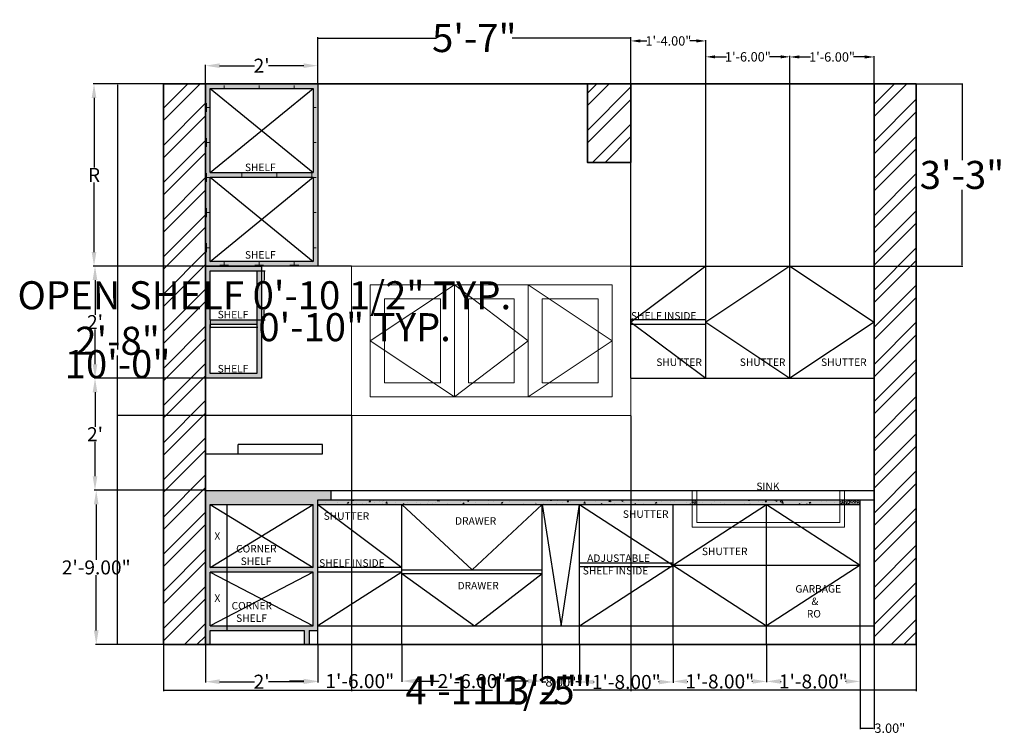
# Model space of a CAD drawing. Units: inches. Extents: x 14 to 1508, y -30 to 806.
# Tile 3 of 4: x 782 to 993, y 297 to 450. Entities that reach past the tile are written whole.
import ezdxf

# ---------------------------------------------------------------- set-up
doc = ezdxf.new("R2010")
doc.units = ezdxf.units.IN
doc.header["$MEASUREMENT"] = 0
for name, color, linetype, lineweight in [('A-ANNO-DIMS', 6, 'Continuous', 18), ('A-ANNO-TEXT', 7, 'Continuous', 18), ('A-ELEV-CASE-BASE', 7, 'Continuous', 25), ('A-ELEV-CASE-PATT', 8, 'Continuous', 13), ('A-ELEV-CASE-UPPR', 7, 'Continuous', 25), ('A-ELEV-CNTR', 7, 'Continuous', 25), ('A-FLOR-FIXT', 8, 'Continuous', 18), ('A-GLAZ', 4, 'Continuous', 18), ('A-WALL', 7, 'Continuous', 35), ('A-WALL-PATT', 8, 'Continuous', 13)]:
    doc.layers.add(name, color=color, linetype=linetype, lineweight=lineweight)
doc.styles.get("Standard").update_dxf_attribs({"font": 'arial.ttf'})
doc.dimstyles.get("Standard").update_dxf_attribs({"dimtxt": 6, "dimasz": 0.18, "dimexe": 0.18, "dimexo": 0.0625, "dimgap": 0.09, "dimtad": 0, "dimtih": 1, "dimtoh": 1, "dimzin": 0, "dimdsep": 46, "dimlunit": 3, "dimtxsty": 'Standard', "dimcen": 0.09, "dimadec": 0, "dimazin": 0, "dimtfac": 1, "dimtofl": 0, "dimtmove": 0, "dimatfit": 3, "dimfxl": 1, "dimtolj": 1, "dimtzin": 0, "dimarcsym": 0})
pattern_1 = [(50, (0, 0), (0.35863009, -0.03137607), [0.0375, -0.4125]), (355, (0, 0), (-0.06937567, 0.37609607), [0.03, -0.33]), (100.451444, (0.0299, -0.0026), (0.28925442, 0.34472), [0.0318701, -0.35057106]), (46.1842, (0, 0.1), (0.53362067, -0.08275964), [0.05625, -0.61875]), (96.635635, (0.04447, 0.0931), (0.46733097, 0.4870593), [0.04780517, -0.52585688]), (351.184164, (0, 0.1), (0.46733097, 0.4870593), [0.045, -0.495]), (21, (0.05, 0.075), (0.29845353, -0.201309445), [0.0375, -0.4125]), (326, (0.05, 0.075), (0.12165767, 0.36257502), [0.03, -0.33]), (71.451445, (0.07487, 0.05822), (0.42011119, 0.16126558), [0.0318701, -0.35057106]), (37.5, (0, 0), (0.006079928, 0.166446927), [0, -0.326, 0, -0.335, 0, -0.33125]), (7.5, (0, 0), (0.13153477, 0.197205856), [0, -0.191, 0, -0.3185, 0, -0.12625]), (327.5, (-0.1115, 0), (0.266911218, -0.011277436), [0, -0.125, 0, -0.39, 0, -0.5175]), (317.5, (-0.1615, 0), (0.291593085, 0.05005249), [0, -0.1625, 0, -0.259, 0, -0.3675])]
pattern_2 = [(50, (0, 0), (3.586301, -0.313761), [0.375, -4.125]), (355, (0, 0), (-0.693757, 3.760961), [0.3, -3.3]), (100.45144, (0.299, -0.026), (2.892544, 3.4472), [0.318701, -3.50571]), (46.1842, (0, 1), (5.336207, -0.827596), [0.5625, -6.1875]), (96.63564, (0.4447, 0.931), (4.67331, 4.870593), [0.478052, -5.25857]), (351.18416, (0, 1), (4.67331, 4.870593), [0.45, -4.95]), (21, (0.5, 0.75), (2.984535, -2.0130945), [0.375, -4.125]), (326, (0.5, 0.75), (1.216577, 3.62575), [0.3, -3.3]), (71.45144, (0.7487, 0.5822), (4.201112, 1.612656), [0.318701, -3.50571]), (37.5, (0, 0), (0.0607993, 1.6644693), [0, -3.26, 0, -3.35, 0, -3.3125]), (7.5, (0, 0), (1.3153477, 1.9720586), [0, -1.91, 0, -3.185, 0, -1.2625]), (327.5, (-1.115, 0), (2.6691122, -0.1127744), [0, -1.25, 0, -3.9, 0, -5.175]), (317.5, (-1.615, 0), (2.915931, 0.500525), [0, -1.625, 0, -2.59, 0, -3.675])]

# ---------------------------------------------------------------- blocks, each defined once
blk = doc.blocks.new('*D39')
at = {"layer": 'A-ANNO-DIMS', "color": 0, "lineweight": -2, "transparency": 16777216}
for p, q in [((821.95, 436.38), (821.95, 440.39)), ((845.95, 436.38), (845.95, 440.39))]:
    blk.add_line(p, q, dxfattribs=at)
at = {"layer": 'A-ANNO-DIMS', "color": 0, "lineweight": -3, "transparency": 16777216}
for p, q in [((824.95, 440.21), (832.45, 440.21)), ((842.95, 440.21), (835.45, 440.21))]:
    blk.add_line(p, q, dxfattribs=at)
at = {"layer": 'A-ANNO-DIMS', "color": 0, "transparency": 16777216}
for points in [[(824.95, 440.71), (824.95, 439.71), (821.95, 440.21)], [(842.95, 440.71), (842.95, 439.71), (845.95, 440.21)]]:
    blk.add_solid(points, dxfattribs=at)
at = {"layer": 'Defpoints', "color": 0, "transparency": 16777216}
for p in [(845.95, 440.21), (821.95, 436.32), (845.95, 436.32)]:
    blk.add_point(p, dxfattribs=at)
at = {"layer": 'A-ANNO-DIMS', "color": 0, "transparency": 16777216, "insert": (833.95, 440.21), "char_height": 3, "attachment_point": 5}
blk.add_mtext("\\A1;2'", dxfattribs=at)
blk = doc.blocks.new('*D40')
at = {"layer": 'A-ANNO-DIMS', "color": 0, "lineweight": -2, "transparency": 16777216}
for p, q in [((821.89, 436.32), (797.93, 436.32)), ((821.89, 397.32), (797.93, 397.32))]:
    blk.add_line(p, q, dxfattribs=at)
at = {"layer": 'A-ANNO-DIMS', "color": 0, "lineweight": -3, "transparency": 16777216}
for p, q in [((798.11, 433.32), (798.11, 418.41)), ((798.11, 400.32), (798.11, 415.23))]:
    blk.add_line(p, q, dxfattribs=at)
at = {"layer": 'A-ANNO-DIMS', "color": 0, "transparency": 16777216}
for points in [[(797.61, 433.32), (798.61, 433.32), (798.11, 436.32)], [(797.61, 400.32), (798.61, 400.32), (798.11, 397.32)]]:
    blk.add_solid(points, dxfattribs=at)
at = {"layer": 'Defpoints', "color": 0, "transparency": 16777216}
for p in [(798.11, 436.32), (821.95, 436.32), (821.95, 397.32)]:
    blk.add_point(p, dxfattribs=at)
at = {"layer": 'A-ANNO-DIMS', "color": 0, "transparency": 16777216, "insert": (798.11, 416.82), "char_height": 3, "attachment_point": 5}
blk.add_mtext('\\A1;R', dxfattribs=at)
blk = doc.blocks.new('*D41')
at = {"layer": 'A-ANNO-DIMS', "color": 0, "lineweight": -2, "transparency": 16777216}
for p, q in [((821.89, 397.32), (798.14, 397.32)), ((821.89, 373.32), (798.14, 373.32))]:
    blk.add_line(p, q, dxfattribs=at)
at = {"layer": 'A-ANNO-DIMS', "color": 0, "lineweight": -3, "transparency": 16777216}
for p, q in [((798.32, 394.32), (798.32, 386.91)), ((798.32, 376.32), (798.32, 383.72))]:
    blk.add_line(p, q, dxfattribs=at)
at = {"layer": 'A-ANNO-DIMS', "color": 0, "transparency": 16777216}
for points in [[(797.82, 394.32), (798.82, 394.32), (798.32, 397.32)], [(797.82, 376.32), (798.82, 376.32), (798.32, 373.32)]]:
    blk.add_solid(points, dxfattribs=at)
at = {"layer": 'Defpoints', "color": 0, "transparency": 16777216}
for p in [(821.95, 397.32), (798.32, 373.32), (821.95, 373.32)]:
    blk.add_point(p, dxfattribs=at)
at = {"layer": 'A-ANNO-DIMS', "color": 0, "transparency": 16777216, "insert": (798.32, 385.32), "char_height": 3, "attachment_point": 5}
blk.add_mtext("\\A1;2'", dxfattribs=at)
blk = doc.blocks.new('*D42')
at = {"layer": 'A-ANNO-DIMS', "color": 0, "lineweight": -2, "transparency": 16777216}
for p, q in [((821.89, 373.32), (798.14, 373.32)), ((821.89, 349.32), (798.14, 349.32))]:
    blk.add_line(p, q, dxfattribs=at)
at = {"layer": 'A-ANNO-DIMS', "color": 0, "lineweight": -3, "transparency": 16777216}
for p, q in [((798.32, 370.32), (798.32, 362.91)), ((798.32, 352.32), (798.32, 359.72))]:
    blk.add_line(p, q, dxfattribs=at)
at = {"layer": 'A-ANNO-DIMS', "color": 0, "transparency": 16777216}
for points in [[(797.82, 370.32), (798.82, 370.32), (798.32, 373.32)], [(797.82, 352.32), (798.82, 352.32), (798.32, 349.32)]]:
    blk.add_solid(points, dxfattribs=at)
at = {"layer": 'Defpoints', "color": 0, "transparency": 16777216}
for p in [(821.95, 373.32), (798.32, 349.32), (821.95, 349.32)]:
    blk.add_point(p, dxfattribs=at)
at = {"layer": 'A-ANNO-DIMS', "color": 0, "transparency": 16777216, "insert": (798.32, 361.32), "char_height": 3, "attachment_point": 5}
blk.add_mtext("\\A1;2'", dxfattribs=at)
blk = doc.blocks.new('*D43')
at = {"layer": 'A-ANNO-DIMS', "color": 0, "lineweight": -2, "transparency": 16777216}
for p, q in [((812.89, 349.32), (798.4, 349.32)), ((812.89, 316.32), (798.4, 316.32))]:
    blk.add_line(p, q, dxfattribs=at)
at = {"layer": 'A-ANNO-DIMS', "color": 0, "lineweight": -3, "transparency": 16777216}
for p, q in [((798.58, 346.32), (798.58, 334.44)), ((798.58, 319.32), (798.58, 331.19))]:
    blk.add_line(p, q, dxfattribs=at)
at = {"layer": 'A-ANNO-DIMS', "color": 0, "transparency": 16777216}
for points in [[(798.08, 346.32), (799.08, 346.32), (798.58, 349.32)], [(798.08, 319.32), (799.08, 319.32), (798.58, 316.32)]]:
    blk.add_solid(points, dxfattribs=at)
at = {"layer": 'Defpoints', "color": 0, "transparency": 16777216}
for p in [(812.95, 349.32), (798.58, 316.32), (812.95, 316.32)]:
    blk.add_point(p, dxfattribs=at)
at = {"layer": 'A-ANNO-DIMS', "color": 0, "transparency": 16777216, "insert": (798.58, 332.82), "char_height": 3, "attachment_point": 5}
blk.add_mtext('\\A1;2\'-9.00"', dxfattribs=at)
blk = doc.blocks.new('*D44')
at = {"layer": 'A-ANNO-DIMS', "color": 0, "lineweight": -2, "transparency": 16777216}
for p, q in [((821.95, 316.25), (821.95, 308.18)), ((845.95, 316.25), (845.95, 308.18))]:
    blk.add_line(p, q, dxfattribs=at)
at = {"layer": 'A-ANNO-DIMS', "color": 0, "lineweight": -3, "transparency": 16777216}
for p, q in [((824.95, 308.36), (832.45, 308.36)), ((842.95, 308.36), (835.45, 308.36))]:
    blk.add_line(p, q, dxfattribs=at)
at = {"layer": 'A-ANNO-DIMS', "color": 0, "transparency": 16777216}
for points in [[(824.95, 308.86), (824.95, 307.86), (821.95, 308.36)], [(842.95, 308.86), (842.95, 307.86), (845.95, 308.36)]]:
    blk.add_solid(points, dxfattribs=at)
at = {"layer": 'Defpoints', "color": 0, "transparency": 16777216}
for p in [(821.95, 316.32), (845.95, 316.32), (845.95, 308.36)]:
    blk.add_point(p, dxfattribs=at)
at = {"layer": 'A-ANNO-DIMS', "color": 0, "transparency": 16777216, "insert": (833.95, 308.36), "char_height": 3, "attachment_point": 5}
blk.add_mtext("\\A1;2'", dxfattribs=at)
blk = doc.blocks.new('*D45')
at = {"layer": 'A-ANNO-DIMS', "color": 0, "lineweight": -2, "transparency": 16777216}
for p, q in [((845.95, 316.25), (845.95, 308.31)), ((863.95, 316.25), (863.95, 308.31))]:
    blk.add_line(p, q, dxfattribs=at)
at = {"layer": 'A-ANNO-DIMS', "color": 0, "lineweight": -3, "transparency": 16777216}
for p, q in [((842.95, 308.49), (839.95, 308.49)), ((866.95, 308.49), (869.95, 308.49))]:
    blk.add_line(p, q, dxfattribs=at)
at = {"layer": 'A-ANNO-DIMS', "color": 0, "transparency": 16777216}
for points in [[(842.95, 308.99), (842.95, 307.99), (845.95, 308.49)], [(866.95, 308.99), (866.95, 307.99), (863.95, 308.49)]]:
    blk.add_solid(points, dxfattribs=at)
at = {"layer": 'Defpoints', "color": 0, "transparency": 16777216}
for p in [(845.95, 316.32), (863.95, 316.32), (863.95, 308.49)]:
    blk.add_point(p, dxfattribs=at)
at = {"layer": 'A-ANNO-DIMS', "color": 0, "transparency": 16777216, "insert": (854.95, 308.49), "char_height": 3, "attachment_point": 5}
blk.add_mtext('\\A1;1\'-6.00"', dxfattribs=at)
blk = doc.blocks.new('*D46')
at = {"layer": 'A-ANNO-DIMS', "color": 0, "lineweight": -2, "transparency": 16777216}
for p, q in [((863.95, 316.25), (863.95, 308.31)), ((893.95, 316.25), (893.95, 308.31))]:
    blk.add_line(p, q, dxfattribs=at)
at = {"layer": 'A-ANNO-DIMS', "color": 0, "lineweight": -3, "transparency": 16777216}
for p, q in [((866.95, 308.49), (871.93, 308.49)), ((890.95, 308.49), (885.97, 308.49))]:
    blk.add_line(p, q, dxfattribs=at)
at = {"layer": 'A-ANNO-DIMS', "color": 0, "transparency": 16777216}
for points in [[(866.95, 308.99), (866.95, 307.99), (863.95, 308.49)], [(890.95, 308.99), (890.95, 307.99), (893.95, 308.49)]]:
    blk.add_solid(points, dxfattribs=at)
at = {"layer": 'Defpoints', "color": 0, "transparency": 16777216}
for p in [(863.95, 316.32), (893.95, 316.32), (893.95, 308.49)]:
    blk.add_point(p, dxfattribs=at)
at = {"layer": 'A-ANNO-DIMS', "color": 0, "transparency": 16777216, "insert": (878.95, 308.49), "char_height": 3, "attachment_point": 5}
blk.add_mtext('\\A1;2\'-6.00"', dxfattribs=at)
blk = doc.blocks.new('*D47')
at = {"layer": 'A-ANNO-DIMS', "color": 0, "lineweight": -2, "transparency": 16777216}
for p, q in [((901.95, 316.25), (901.95, 308.12)), ((921.95, 316.25), (921.95, 308.12))]:
    blk.add_line(p, q, dxfattribs=at)
at = {"layer": 'A-ANNO-DIMS', "color": 0, "lineweight": -3, "transparency": 16777216}
for p, q in [((904.95, 308.3), (905.1, 308.3)), ((918.95, 308.3), (918.8, 308.3))]:
    blk.add_line(p, q, dxfattribs=at)
at = {"layer": 'A-ANNO-DIMS', "color": 0, "transparency": 16777216}
for points in [[(904.95, 308.8), (904.95, 307.8), (901.95, 308.3)], [(918.95, 308.8), (918.95, 307.8), (921.95, 308.3)]]:
    blk.add_solid(points, dxfattribs=at)
at = {"layer": 'Defpoints', "color": 0, "transparency": 16777216}
for p in [(901.95, 316.32), (921.95, 316.32), (921.95, 308.3)]:
    blk.add_point(p, dxfattribs=at)
at = {"layer": 'A-ANNO-DIMS', "color": 0, "transparency": 16777216, "insert": (911.95, 308.3), "char_height": 3, "attachment_point": 5}
blk.add_mtext('\\A1;1\'-8.00"', dxfattribs=at)
blk = doc.blocks.new('*D48')
at = {"layer": 'A-ANNO-DIMS', "color": 0, "lineweight": -2, "transparency": 16777216}
for p, q in [((893.95, 316.25), (893.95, 308.12)), ((901.95, 316.25), (901.95, 308.12)), ((894.13, 308.3), (894.77, 308.3)), ((901.77, 308.3), (901.13, 308.3))]:
    blk.add_line(p, q, dxfattribs=at)
at = {"layer": 'A-ANNO-DIMS', "color": 0, "transparency": 16777216}
for points in [[(894.13, 308.33), (894.13, 308.27), (893.95, 308.3)], [(901.77, 308.33), (901.77, 308.27), (901.95, 308.3)]]:
    blk.add_solid(points, dxfattribs=at)
at = {"layer": 'Defpoints', "color": 0, "transparency": 16777216}
for p in [(893.95, 316.32), (901.95, 316.32), (901.95, 308.3)]:
    blk.add_point(p, dxfattribs=at)
at = {"layer": 'A-ANNO-DIMS', "color": 0, "transparency": 16777216, "insert": (897.95, 308.3), "char_height": 2, "attachment_point": 5}
blk.add_mtext('\\A1;8.00"', dxfattribs=at)
blk = doc.blocks.new('*D49')
at = {"layer": 'A-ANNO-DIMS', "color": 0, "lineweight": -2, "transparency": 16777216}
for p, q in [((921.95, 316.25), (921.95, 308.24)), ((941.95, 316.25), (941.95, 308.24))]:
    blk.add_line(p, q, dxfattribs=at)
at = {"layer": 'A-ANNO-DIMS', "color": 0, "lineweight": -3, "transparency": 16777216}
for p, q in [((924.95, 308.42), (925.1, 308.42)), ((938.95, 308.42), (938.8, 308.42))]:
    blk.add_line(p, q, dxfattribs=at)
at = {"layer": 'A-ANNO-DIMS', "color": 0, "transparency": 16777216}
for points in [[(924.95, 308.92), (924.95, 307.92), (921.95, 308.42)], [(938.95, 308.92), (938.95, 307.92), (941.95, 308.42)]]:
    blk.add_solid(points, dxfattribs=at)
at = {"layer": 'Defpoints', "color": 0, "transparency": 16777216}
for p in [(921.95, 316.32), (941.95, 316.32), (941.95, 308.42)]:
    blk.add_point(p, dxfattribs=at)
at = {"layer": 'A-ANNO-DIMS', "color": 0, "transparency": 16777216, "insert": (931.95, 308.42), "char_height": 3, "attachment_point": 5}
blk.add_mtext('\\A1;1\'-8.00"', dxfattribs=at)
blk = doc.blocks.new('*D50')
at = {"layer": 'A-ANNO-DIMS', "color": 0, "lineweight": -2, "transparency": 16777216}
for p, q in [((941.95, 316.25), (941.95, 308.24)), ((961.95, 316.25), (961.95, 308.24))]:
    blk.add_line(p, q, dxfattribs=at)
at = {"layer": 'A-ANNO-DIMS', "color": 0, "lineweight": -3, "transparency": 16777216}
for p, q in [((944.95, 308.42), (945.1, 308.42)), ((958.95, 308.42), (958.8, 308.42))]:
    blk.add_line(p, q, dxfattribs=at)
at = {"layer": 'A-ANNO-DIMS', "color": 0, "transparency": 16777216}
for points in [[(944.95, 308.92), (944.95, 307.92), (941.95, 308.42)], [(958.95, 308.92), (958.95, 307.92), (961.95, 308.42)]]:
    blk.add_solid(points, dxfattribs=at)
at = {"layer": 'Defpoints', "color": 0, "transparency": 16777216}
for p in [(941.95, 316.32), (961.95, 316.32), (961.95, 308.42)]:
    blk.add_point(p, dxfattribs=at)
at = {"layer": 'A-ANNO-DIMS', "color": 0, "transparency": 16777216, "insert": (951.95, 308.42), "char_height": 3, "attachment_point": 5}
blk.add_mtext('\\A1;1\'-8.00"', dxfattribs=at)
blk = doc.blocks.new('*D51')
at = {"layer": 'A-ANNO-DIMS', "color": 0, "lineweight": -2, "transparency": 16777216}
for p, q in [((961.95, 316.25), (961.95, 298.23)), ((964.95, 316.25), (964.95, 298.23)), ((962.13, 298.41), (964.77, 298.41)), ((964.95, 298.41), (965.13, 298.41))]:
    blk.add_line(p, q, dxfattribs=at)
at = {"layer": 'A-ANNO-DIMS', "color": 0, "transparency": 16777216}
for points in [[(962.13, 298.44), (962.13, 298.38), (961.95, 298.41)], [(964.77, 298.44), (964.77, 298.38), (964.95, 298.41)]]:
    blk.add_solid(points, dxfattribs=at)
at = {"layer": 'Defpoints', "color": 0, "transparency": 16777216}
for p in [(961.95, 316.32), (964.95, 316.32), (964.95, 298.41)]:
    blk.add_point(p, dxfattribs=at)
at = {"layer": 'A-ANNO-DIMS', "color": 0, "transparency": 16777216, "insert": (968.31, 298.41), "char_height": 2, "attachment_point": 5}
blk.add_mtext('\\A1;3.00"', dxfattribs=at)
blk = doc.blocks.new('*D52')
at = {"layer": 'A-ANNO-DIMS', "color": 0, "lineweight": -2, "transparency": 16777216}
for p, q in [((912.95, 436.38), (912.95, 445.68)), ((914.95, 445.5), (916.35, 445.5)), ((926.95, 445.5), (925.55, 445.5)), ((928.95, 436.38), (928.95, 445.68))]:
    blk.add_line(p, q, dxfattribs=at)
at = {"layer": 'A-ANNO-DIMS', "color": 0, "transparency": 16777216}
for points in [[(914.95, 445.84), (914.95, 445.17), (912.95, 445.5)], [(926.95, 445.84), (926.95, 445.17), (928.95, 445.5)]]:
    blk.add_solid(points, dxfattribs=at)
at = {"layer": 'Defpoints', "color": 0, "transparency": 16777216}
for p in [(928.95, 445.5), (912.95, 436.32), (928.95, 436.32)]:
    blk.add_point(p, dxfattribs=at)
at = {"layer": 'A-ANNO-DIMS', "color": 0, "transparency": 16777216, "insert": (920.95, 445.5), "char_height": 2, "attachment_point": 5}
blk.add_mtext('\\A1;1\'-4.00"', dxfattribs=at)
blk = doc.blocks.new('*D53')
at = {"layer": 'A-ANNO-DIMS', "color": 0, "lineweight": -2, "transparency": 16777216}
for p, q in [((928.95, 436.38), (928.95, 442.28)), ((946.95, 436.38), (946.95, 442.28)), ((930.95, 442.1), (933.35, 442.1)), ((944.95, 442.1), (942.55, 442.1))]:
    blk.add_line(p, q, dxfattribs=at)
at = {"layer": 'A-ANNO-DIMS', "color": 0, "transparency": 16777216}
for points in [[(930.95, 442.43), (930.95, 441.76), (928.95, 442.1)], [(944.95, 442.43), (944.95, 441.76), (946.95, 442.1)]]:
    blk.add_solid(points, dxfattribs=at)
at = {"layer": 'Defpoints', "color": 0, "transparency": 16777216}
for p in [(946.95, 442.1), (928.95, 436.32), (946.95, 436.32)]:
    blk.add_point(p, dxfattribs=at)
at = {"layer": 'A-ANNO-DIMS', "color": 0, "transparency": 16777216, "insert": (937.95, 442.1), "char_height": 2, "attachment_point": 5}
blk.add_mtext('\\A1;1\'-6.00"', dxfattribs=at)
blk = doc.blocks.new('*D54')
at = {"layer": 'A-ANNO-DIMS', "color": 0, "lineweight": -2, "transparency": 16777216}
for p, q in [((946.95, 436.38), (946.95, 442.25)), ((964.95, 436.38), (964.95, 442.25)), ((948.95, 442.07), (951.35, 442.07)), ((962.95, 442.07), (960.55, 442.07))]:
    blk.add_line(p, q, dxfattribs=at)
at = {"layer": 'A-ANNO-DIMS', "color": 0, "transparency": 16777216}
for points in [[(948.95, 442.41), (948.95, 441.74), (946.95, 442.07)], [(962.95, 442.41), (962.95, 441.74), (964.95, 442.07)]]:
    blk.add_solid(points, dxfattribs=at)
at = {"layer": 'Defpoints', "color": 0, "transparency": 16777216}
for p in [(964.95, 442.07), (946.95, 436.32), (964.95, 436.32)]:
    blk.add_point(p, dxfattribs=at)
at = {"layer": 'A-ANNO-DIMS', "color": 0, "transparency": 16777216, "insert": (955.95, 442.07), "char_height": 2, "attachment_point": 5}
blk.add_mtext('\\A1;1\'-6.00"', dxfattribs=at)
blk = doc.blocks.new('CAB-SHELF-FRONT-10IN')
blk.add_line((0, 0), (10, 0))
blk.add_lwpolyline([(0, 0), (0, 10.5), (10, 10.5), (10, 0)])
blk = doc.blocks.new('*D93')
at = {"layer": 'A-ANNO-DIMS', "color": 0, "lineweight": -2, "transparency": 16777216}
for p, q in [((833.01, 396.32), (834.71, 396.32)), ((834.53, 396.14), (834.53, 394.26)), ((834.53, 386), (834.53, 387.87)), ((833.01, 385.82), (834.71, 385.82))]:
    blk.add_line(p, q, dxfattribs=at)
at = {"layer": 'A-ANNO-DIMS', "color": 0, "transparency": 16777216}
for points in [[(834.5, 396.14), (834.56, 396.14), (834.53, 396.32)], [(834.5, 386), (834.56, 386), (834.53, 385.82)]]:
    blk.add_solid(points, dxfattribs=at)
at = {"layer": 'Defpoints', "color": 0, "transparency": 16777216}
for p in [(832.95, 396.32), (834.53, 396.32), (832.95, 385.82)]:
    blk.add_point(p, dxfattribs=at)
at = {"layer": 'A-ANNO-DIMS', "color": 0, "transparency": 16777216, "insert": (834.53, 391.07), "char_height": 6, "attachment_point": 5}
blk.add_mtext('\\A1;OPEN SHELF 0\'-10 1/2" TYP.', dxfattribs=at)
blk = doc.blocks.new('*D94')
at = {"layer": 'A-ANNO-DIMS', "color": 0, "lineweight": -2, "transparency": 16777216}
for p, q in [((822.95, 385.75), (822.95, 384.06)), ((832.95, 385.75), (832.95, 384.06)), ((823.13, 384.24), (832.77, 384.24)), ((832.95, 384.24), (833.13, 384.24))]:
    blk.add_line(p, q, dxfattribs=at)
at = {"layer": 'A-ANNO-DIMS', "color": 0, "transparency": 16777216}
for points in [[(823.13, 384.27), (823.13, 384.21), (822.95, 384.24)], [(832.77, 384.27), (832.77, 384.21), (832.95, 384.24)]]:
    blk.add_solid(points, dxfattribs=at)
at = {"layer": 'Defpoints', "color": 0, "transparency": 16777216}
for p in [(822.95, 385.82), (832.95, 385.82), (832.95, 384.24)]:
    blk.add_point(p, dxfattribs=at)
at = {"layer": 'A-ANNO-DIMS', "color": 0, "transparency": 16777216, "insert": (853.84, 384.24), "char_height": 6, "attachment_point": 5}
blk.add_mtext('\\A1;0\'-10" TYP.', dxfattribs=at)
blk = doc.blocks.new('*D103')
at = {"layer": 'A-ANNO-DIMS', "color": 0, "lineweight": -2, "transparency": 16777216}
for p, q in [((812.95, 316.25), (812.95, 306.34)), ((973.95, 316.25), (973.95, 306.34)), ((813.13, 306.52), (883.34, 306.52)), ((973.77, 306.52), (903.56, 306.52))]:
    blk.add_line(p, q, dxfattribs=at)
at = {"layer": 'A-ANNO-DIMS', "color": 0, "transparency": 16777216}
for points in [[(813.13, 306.55), (813.13, 306.49), (812.95, 306.52)], [(973.77, 306.55), (973.77, 306.49), (973.95, 306.52)]]:
    blk.add_solid(points, dxfattribs=at)
at = {"layer": 'Defpoints', "color": 0, "transparency": 16777216}
for p in [(812.95, 316.32), (973.95, 316.32), (812.95, 306.52)]:
    blk.add_point(p, dxfattribs=at)
at = {"layer": 'A-ANNO-DIMS', "color": 0, "transparency": 16777216, "insert": (893.45, 306.52), "char_height": 6, "attachment_point": 5}
blk.add_mtext('\\A1;13\'-5"', dxfattribs=at)
blk = doc.blocks.new('*D104')
at = {"layer": 'A-ANNO-DIMS', "color": 0, "lineweight": -2, "transparency": 16777216}
for p, q in [((812.89, 436.32), (802.97, 436.32)), ((803.15, 436.14), (803.15, 379.47)), ((803.15, 316.5), (803.15, 373.16)), ((812.89, 316.32), (802.97, 316.32))]:
    blk.add_line(p, q, dxfattribs=at)
at = {"layer": 'A-ANNO-DIMS', "color": 0, "transparency": 16777216}
for points in [[(803.12, 436.14), (803.18, 436.14), (803.15, 436.32)], [(803.12, 316.5), (803.18, 316.5), (803.15, 316.32)]]:
    blk.add_solid(points, dxfattribs=at)
at = {"layer": 'Defpoints', "color": 0, "transparency": 16777216}
for p in [(803.15, 436.32), (812.95, 436.32), (812.95, 316.32)]:
    blk.add_point(p, dxfattribs=at)
at = {"layer": 'A-ANNO-DIMS', "color": 0, "transparency": 16777216, "insert": (803.15, 376.32), "char_height": 6, "attachment_point": 5}
blk.add_mtext('\\A1;10\'-0"', dxfattribs=at)
blk = doc.blocks.new('*D105')
at = {"layer": 'A-ANNO-DIMS', "color": 0, "lineweight": -2, "transparency": 16777216}
for p, q in [((853.2, 365.27), (853.2, 306.34)), ((912.95, 365.27), (912.95, 306.34)), ((853.38, 306.52), (865.57, 306.52)), ((912.77, 306.52), (900.58, 306.52))]:
    blk.add_line(p, q, dxfattribs=at)
at = {"layer": 'A-ANNO-DIMS', "color": 0, "transparency": 16777216}
for points in [[(853.38, 306.55), (853.38, 306.49), (853.2, 306.52)], [(912.77, 306.55), (912.77, 306.49), (912.95, 306.52)]]:
    blk.add_solid(points, dxfattribs=at)
at = {"layer": 'Defpoints', "color": 0, "transparency": 16777216}
for p in [(853.2, 365.34), (912.95, 365.34), (912.95, 306.52)]:
    blk.add_point(p, dxfattribs=at)
at = {"layer": 'A-ANNO-DIMS', "color": 0, "transparency": 16777216, "insert": (883.08, 306.52), "char_height": 6, "attachment_point": 5}
blk.add_mtext('\\A1;4\'-11 1/2"', dxfattribs=at)
blk = doc.blocks.new('*D106')
at = {"layer": 'A-ANNO-DIMS', "color": 0, "lineweight": -2, "transparency": 16777216}
for p, q in [((853.14, 397.32), (802.97, 397.32)), ((803.15, 397.14), (803.15, 384.48)), ((803.15, 365.52), (803.15, 378.17)), ((853.14, 365.34), (802.97, 365.34))]:
    blk.add_line(p, q, dxfattribs=at)
at = {"layer": 'A-ANNO-DIMS', "color": 0, "transparency": 16777216}
for points in [[(803.12, 397.14), (803.18, 397.14), (803.15, 397.32)], [(803.12, 365.52), (803.18, 365.52), (803.15, 365.34)]]:
    blk.add_solid(points, dxfattribs=at)
at = {"layer": 'Defpoints', "color": 0, "transparency": 16777216}
for p in [(803.15, 397.32), (853.2, 397.32), (853.2, 365.34)]:
    blk.add_point(p, dxfattribs=at)
at = {"layer": 'A-ANNO-DIMS', "color": 0, "transparency": 16777216, "insert": (803.15, 381.33), "char_height": 6, "attachment_point": 5}
blk.add_mtext('\\A1;2\'-8"', dxfattribs=at)
blk = doc.blocks.new('*D107')
at = {"layer": 'A-ANNO-DIMS', "color": 0, "lineweight": -2, "transparency": 16777216}
for p, q in [((845.95, 436.38), (845.95, 446.3)), ((846.13, 446.12), (871.39, 446.12)), ((912.77, 446.12), (887.52, 446.12)), ((912.95, 436.38), (912.95, 446.3))]:
    blk.add_line(p, q, dxfattribs=at)
at = {"layer": 'A-ANNO-DIMS', "color": 0, "transparency": 16777216}
for points in [[(846.13, 446.15), (846.13, 446.09), (845.95, 446.12)], [(912.77, 446.15), (912.77, 446.09), (912.95, 446.12)]]:
    blk.add_solid(points, dxfattribs=at)
at = {"layer": 'Defpoints', "color": 0, "transparency": 16777216}
for p in [(912.95, 446.12), (845.95, 436.32), (912.95, 436.32)]:
    blk.add_point(p, dxfattribs=at)
at = {"layer": 'A-ANNO-DIMS', "color": 0, "transparency": 16777216, "insert": (879.45, 446.12), "char_height": 6, "attachment_point": 5}
blk.add_mtext('\\A1;5\'-7"', dxfattribs=at)
blk = doc.blocks.new('*D108')
at = {"layer": 'A-ANNO-DIMS', "color": 0, "lineweight": -2, "transparency": 16777216}
for p, q in [((965.01, 436.32), (983.93, 436.32)), ((983.75, 436.14), (983.75, 419.97)), ((983.75, 397.5), (983.75, 413.66)), ((965.01, 397.32), (983.93, 397.32))]:
    blk.add_line(p, q, dxfattribs=at)
at = {"layer": 'A-ANNO-DIMS', "color": 0, "transparency": 16777216}
for points in [[(983.72, 436.14), (983.78, 436.14), (983.75, 436.32)], [(983.72, 397.5), (983.78, 397.5), (983.75, 397.32)]]:
    blk.add_solid(points, dxfattribs=at)
at = {"layer": 'Defpoints', "color": 0, "transparency": 16777216}
for p in [(964.95, 436.32), (983.75, 436.32), (964.95, 397.32)]:
    blk.add_point(p, dxfattribs=at)
at = {"layer": 'A-ANNO-DIMS', "color": 0, "transparency": 16777216, "insert": (983.75, 416.82), "char_height": 6, "attachment_point": 5}
blk.add_mtext('\\A1;3\'-3"', dxfattribs=at)

msp = doc.modelspace()

# ---------------------------------------------------------------- hatches: boundary and pattern name
at = {"layer": 'A-ELEV-CASE-PATT'}
h = msp.add_hatch(color=256, dxfattribs=at)
h.dxf.hatch_style = 1
h.paths.add_polyline_path([(845.951, 436.316), (821.951, 436.316), (821.951, 397.316), (845.951, 397.316)])
h.paths.add_polyline_path([(822.951, 435.316), (844.951, 435.316), (844.951, 417.316), (822.951, 417.316)], flags=16)
h.paths.add_polyline_path([(822.951, 416.316), (844.951, 416.316), (844.951, 398.316), (822.951, 398.316)], flags=16)
h.paths.add_polyline_path([(833.951, 397.316), (821.951, 397.316), (821.951, 373.316), (833.951, 373.316)])
h.paths.add_polyline_path([(832.951, 385.816), (822.951, 385.816), (822.951, 396.316), (832.951, 396.316)], flags=16)
h.paths.add_polyline_path([(832.951, 384.816), (832.951, 374.316), (822.951, 374.316), (822.951, 384.816)], flags=16)
h = msp.add_hatch(dxfattribs=at)
h.set_pattern_fill('CROSS', color=256, scale=15)
h.paths.add_polyline_path([(845.951, 436.316), (821.951, 436.316), (821.951, 397.316), (833.951, 397.316), (845.951, 397.316)])
h.paths.add_polyline_path([(822.951, 398.316), (822.951, 416.316), (844.951, 416.316), (844.951, 398.316)], flags=16)
h.paths.add_polyline_path([(822.951, 417.316), (822.951, 435.316), (844.951, 435.316), (844.951, 417.316)], flags=16)
h.paths.add_polyline_path([(829.888, 416.743), (837.892, 416.743), (837.892, 420.04), (829.888, 420.04)], flags=24)
h.paths.add_polyline_path([(829.888, 398.014), (837.892, 398.014), (837.892, 401.312), (829.888, 401.312)], flags=24)
h = msp.add_hatch(color=256, dxfattribs=at)
h.dxf.hatch_style = 1
h.paths.add_polyline_path([(822.951, 331.816), (826.498, 331.816), (826.498, 332.816), (822.951, 332.816), (822.951, 346.316), (844.951, 346.316), (844.951, 332.816), (826.498, 332.816), (826.498, 331.816), (844.951, 331.816), (844.951, 320.316), (826.498, 320.316), (826.498, 319.316), (843.087, 319.316), (843.087, 316.316), (844.087, 316.316), (844.087, 319.316), (845.951, 319.316), (845.951, 347.316), (848.751, 347.316), (848.751, 349.316), (821.951, 349.316), (821.951, 316.316), (822.951, 316.316), (822.951, 319.316), (826.498, 319.316), (826.498, 320.316), (822.951, 320.316)])
h = msp.add_hatch(dxfattribs=at)
h.set_pattern_fill('AR-CONC', color=256, scale=0.5)
h.set_pattern_definition(pattern_2)
h.paths.add_polyline_path([(926.064, 346.316), (926.064, 347.316), (845.951, 347.316), (845.951, 346.316)])
h = msp.add_hatch(dxfattribs=at)
h.set_pattern_fill('AR-CONC', color=256, scale=0.05)
h.set_pattern_definition(pattern_1)
h.paths.add_polyline_path([(926.064, 346.316), (926.064, 347.316), (845.951, 347.316), (845.951, 346.316)])
h.paths.add_polyline_path([(957.64, 346.316), (957.64, 347.316), (927.064, 347.316), (927.064, 346.316)])
h = msp.add_hatch(dxfattribs=at)
h.set_pattern_fill('AR-CONC', color=256, scale=0.05)
h.set_pattern_definition(pattern_1)
h.paths.add_polyline_path([(926.064, 347.316), (926.064, 346.316), (927.064, 346.316), (927.064, 347.316)])
h = msp.add_hatch(dxfattribs=at)
h.set_pattern_fill('AR-CONC', color=256, scale=0.05)
h.set_pattern_definition(pattern_1)
h.paths.add_polyline_path([(927.064, 347.316), (927.064, 346.316), (957.64, 346.316), (957.64, 347.316)])
h = msp.add_hatch(dxfattribs=at)
h.set_pattern_fill('AR-CONC', color=256, scale=0.5)
h.set_pattern_definition(pattern_2)
h.paths.add_polyline_path([(957.64, 346.316), (957.64, 347.316), (927.064, 347.316), (927.064, 346.316)])
h = msp.add_hatch(dxfattribs=at)
h.set_pattern_fill('AR-CONC', color=256, scale=0.05)
h.set_pattern_definition(pattern_1)
h.paths.add_polyline_path([(958.64, 347.316), (957.64, 347.316), (957.64, 346.316), (958.64, 346.316)])
h = msp.add_hatch(dxfattribs=at)
h.set_pattern_fill('AR-CONC', color=256, scale=0.5)
h.set_pattern_definition(pattern_2)
h.paths.add_polyline_path([(958.64, 347.316), (958.64, 346.316), (961.951, 346.316), (961.951, 347.316)])
h = msp.add_hatch(dxfattribs=at)
h.set_pattern_fill('AR-CONC', color=256, scale=0.5)
h.set_pattern_definition(pattern_2)
h.paths.add_polyline_path([(958.64, 347.316), (958.64, 346.316), (961.951, 346.316), (961.951, 347.316)])
h = msp.add_hatch(dxfattribs=at)
h.set_pattern_fill('AR-CONC', color=256, scale=0.05)
h.set_pattern_definition(pattern_1)
h.paths.add_polyline_path([(961.951, 346.316), (961.951, 347.316), (958.64, 347.316), (958.64, 346.316)])
at = {"layer": 'A-WALL-PATT'}
h = msp.add_hatch(dxfattribs=at)
h.set_pattern_fill('ANSI32', color=256, scale=15)
h.paths.add_polyline_path([(821.951, 436.316), (812.951, 436.316), (812.951, 316.316), (821.951, 316.316)])
h = msp.add_hatch(dxfattribs=at)
h.set_pattern_fill('ANSI32', color=256, scale=15)
h.paths.add_polyline_path([(912.951, 436.316), (903.648, 436.316), (903.648, 419.488), (912.951, 419.488)])
h = msp.add_hatch(dxfattribs=at)
h.set_pattern_fill('ANSI32', color=256, scale=15)
h.paths.add_polyline_path([(973.951, 436.316), (964.951, 436.316), (964.951, 316.316), (973.951, 316.316)])

# ---------------------------------------------------------------- linework, layer by layer
at = {"layer": 'A-ELEV-CASE-BASE'}
for p, q in [((822.951, 332.816), (822.951, 346.316)), ((822.951, 332.816), (844.951, 346.316)), ((822.951, 346.316), (844.951, 332.816)), ((822.951, 346.316), (844.951, 346.316)), ((826.498, 346.316), (826.498, 319.316)), ((844.951, 332.816), (844.951, 346.316)), ((845.951, 316.316), (845.951, 347.316)), ((845.951, 346.316), (863.951, 332.816)), ((863.951, 316.316), (863.951, 346.316)), ((863.951, 346.316), (878.951, 332.31)), ((878.951, 332.31), (893.951, 346.316)), ((893.951, 316.316), (893.951, 346.316)), ((893.951, 346.316), (898.047, 320.316)), ((898.047, 320.316), (901.951, 346.316)), ((901.951, 316.316), (901.951, 346.316)), ((901.951, 346.316), (941.951, 320.316)), ((901.951, 320.316), (941.951, 346.316)), ((921.951, 316.316), (921.951, 346.316)), ((941.951, 316.316), (941.951, 346.316)), ((941.951, 346.316), (961.951, 333.316)), ((961.951, 316.316), (961.951, 347.316)), ((844.951, 332.816), (822.951, 332.816)), ((863.951, 332.816), (845.951, 332.816)), ((921.951, 333.716), (901.951, 333.716)), ((921.951, 332.916), (901.951, 332.916)), ((921.951, 333.316), (961.951, 333.316)), ((961.951, 333.316), (941.951, 320.316)), ((822.951, 320.316), (822.951, 331.816)), ((844.951, 331.816), (822.951, 331.816)), ((822.951, 331.816), (844.951, 320.316)), ((844.951, 331.816), (822.951, 320.316)), ((844.951, 320.316), (844.951, 331.816)), ((863.951, 331.816), (845.951, 331.816)), ((863.951, 331.816), (845.951, 320.316)), ((863.951, 332.31), (893.951, 332.31)), ((863.951, 331.51), (893.951, 331.51)), ((863.951, 331.51), (879.471, 320.316)), ((879.471, 320.316), (893.951, 331.51)), ((822.951, 320.316), (844.951, 320.316)), ((845.951, 320.316), (964.951, 320.316)), ((822.951, 319.316), (843.087, 319.316)), ((822.951, 316.316), (822.951, 319.316)), ((843.087, 319.316), (843.087, 316.316)), ((844.087, 319.316), (844.087, 316.316)), ((844.087, 319.316), (845.951, 319.316))]:
    msp.add_line(p, q, dxfattribs=at)
at = {"layer": 'A-ELEV-CASE-UPPR'}
for p, q in [((912.951, 397.316), (912.951, 436.316)), ((928.951, 373.316), (928.951, 436.316)), ((946.951, 373.316), (946.951, 436.316)), ((822.951, 435.316), (844.951, 417.316)), ((822.951, 417.316), (844.951, 435.316)), ((822.951, 417.316), (844.951, 417.316)), ((822.951, 416.316), (844.951, 416.316)), ((822.951, 416.316), (844.951, 398.316)), ((822.951, 398.316), (844.951, 416.316)), ((912.951, 397.316), (964.951, 397.316)), ((912.951, 373.316), (912.951, 397.316)), ((928.951, 397.316), (912.951, 385.316)), ((946.951, 397.316), (928.951, 385.316)), ((946.951, 397.316), (964.951, 385.316)), ((928.951, 385.816), (912.951, 385.816)), ((912.951, 385.316), (928.951, 373.316)), ((928.951, 384.816), (912.951, 384.816)), ((928.951, 385.316), (946.951, 373.316)), ((964.951, 385.316), (946.951, 373.316)), ((912.951, 373.316), (964.951, 373.316)), ((828.951, 357.16), (828.951, 359.118)), ((846.951, 359.118), (828.951, 359.118)), ((846.951, 357.16), (846.951, 359.118)), ((821.951, 357.16), (828.951, 357.16)), ((828.951, 357.16), (846.951, 357.16))]:
    msp.add_line(p, q, dxfattribs=at)
for points in [[(821.951, 397.316), (821.951, 436.316), (845.951, 436.316)], [(822.951, 417.316), (822.951, 435.316), (844.951, 435.316), (844.951, 417.316)], [(844.951, 416.316), (844.951, 398.316), (822.951, 398.316), (822.951, 416.316)]]:
    msp.add_lwpolyline(points, dxfattribs=at)
for points in [[(821.951, 436.316), (845.951, 436.316), (845.951, 397.316), (821.951, 397.316)], [(821.951, 397.316), (833.951, 397.316), (833.951, 373.316), (821.951, 373.316)]]:
    msp.add_lwpolyline(points, close=True, dxfattribs=at)
at = {"layer": 'A-ELEV-CNTR'}
for p, q in [((821.951, 349.316), (893.951, 349.316)), ((848.751, 349.316), (848.751, 347.316)), ((893.951, 349.316), (964.951, 349.316)), ((845.951, 347.316), (964.951, 347.316)), ((845.951, 346.316), (961.951, 346.316))]:
    msp.add_line(p, q, dxfattribs=at)
at = {"layer": 'A-FLOR-FIXT'}
for p, q in [((926.064, 349.316), (926.064, 341.432)), ((927.064, 349.316), (927.064, 342.432)), ((957.64, 342.432), (957.64, 349.316)), ((958.64, 341.432), (958.64, 349.316)), ((926.064, 341.432), (958.64, 341.432)), ((927.064, 342.432), (957.64, 342.432))]:
    msp.add_line(p, q, dxfattribs=at)
at = {"layer": 'A-GLAZ'}
for p, q in [((875.202, 393.316), (857.202, 381.326)), ((890.951, 381.326), (875.202, 393.316)), ((890.951, 393.316), (908.951, 381.326)), ((857.202, 381.326), (875.202, 369.336)), ((875.202, 369.336), (890.951, 381.326)), ((908.951, 381.326), (890.951, 369.336))]:
    msp.add_line(p, q, dxfattribs=at)
for points in [[(912.951, 397.316), (853.202, 397.316), (853.202, 365.336), (912.951, 365.336)], [(857.202, 393.316), (875.202, 393.316), (875.202, 369.336), (857.202, 369.336)], [(875.202, 393.316), (890.951, 393.316), (890.951, 369.336), (875.202, 369.336)], [(890.951, 393.316), (908.951, 393.316), (908.951, 369.336), (890.951, 369.336)], [(860.202, 390.316), (872.202, 390.316), (872.202, 372.336), (860.202, 372.336)], [(878.202, 390.316), (887.951, 390.316), (887.951, 372.336), (878.202, 372.336)], [(893.951, 390.316), (905.951, 390.316), (905.951, 372.336), (893.951, 372.336)]]:
    msp.add_lwpolyline(points, close=True, dxfattribs=at)
for points in [[(908.951, 393.316), (857.202, 393.316)], [(857.202, 393.316), (857.202, 369.336)], [(875.202, 393.316), (875.202, 369.336)], [(890.951, 369.336), (890.951, 393.316)], [(908.951, 369.336), (908.951, 393.316)], [(857.202, 369.336), (908.951, 369.336)]]:
    msp.add_lwpolyline(points, dxfattribs=at)
at = {"layer": 'A-WALL'}
for p, q in [((812.951, 316.316), (812.951, 436.316)), ((812.951, 436.316), (973.951, 436.316)), ((821.951, 316.316), (821.951, 436.316)), ((964.951, 316.316), (964.951, 436.316)), ((973.951, 316.316), (973.951, 436.316)), ((812.951, 316.316), (973.951, 316.316))]:
    msp.add_line(p, q, dxfattribs=at)
msp.add_lwpolyline([(912.951, 436.316), (903.648, 436.316), (903.648, 419.488), (912.951, 419.488)], close=True, dxfattribs=at)

# ---------------------------------------------------------------- block references
at = {"layer": 'A-ELEV-CASE-UPPR'}
msp.add_blockref('CAB-SHELF-FRONT-10IN', (822.951, 385.816), dxfattribs=at)
at = {"layer": 'A-ELEV-CASE-UPPR', "rotation": 180}
msp.add_blockref('CAB-SHELF-FRONT-10IN', (832.951, 384.816), dxfattribs=at)

# ---------------------------------------------------------------- texts
at = {"layer": 'A-ANNO-TEXT', "char_height": 1.6, "attachment_point": 1}
for s, insert in [('SHELF', (830.388, 419.244)), ('SHELF', (830.388, 400.515)), ('SHELF', (824.55, 387.736)), ('SHELF INSIDE', (912.951, 387.47)), ('\\PSHUTTER', (918.359, 380.209)), ('\\PSHUTTER', (936.221, 380.209)), ('\\PSHUTTER', (953.596, 380.209)), ('SHELF', (824.55, 376.154)), ('SINK', (939.766, 350.962)), ('SHUTTER', (847.219, 344.618)), ('DRAWER', (875.326, 343.575)), ('SHUTTER', (911.215, 345.031)), ('X', (823.861, 340.339)), ('CORNER\\P  SHELF', (828.502, 337.615)), ('SHUTTER', (928.121, 337.054)), ('ADJUSTABLE', (903.575, 335.601)), ('SHELF INSIDE', (846.259, 334.566)), ('SHELF INSIDE', (902.641, 332.916)), ('DRAWER', (875.859, 329.73)), ('GARBAGE\\P       &\\P     RO', (948.112, 329.034)), ('X', (823.861, 327.048)), ('CORNER\\P  SHELF', (827.529, 325.426))]:
    msp.add_mtext_dynamic_manual_height_columns(s, width=28.12131, gutter_width=1, heights=[0], dxfattribs=dict(at, insert=insert))

# ---------------------------------------------------------------- dimensions: what is measured, and where the dimension line sits
at = {"layer": 'A-ANNO-DIMS'}
for base, p1, p2, override, picture, middle in [((912.951, 446.116), (845.951, 436.316), (912.951, 436.316), {"dimdec": 1, "dimlfac": 1, "dimrnd": 0, "dimzin": 1, "dimdsep": 46, "dimlunit": 4, "dimfrac": 2}, '*D107', (879.451, 446.116)), ((928.951, 445.502), (912.951, 436.316), (928.951, 436.316), {"dimtxt": 2, "dimasz": 2, "dimclrd": 0, "dimclre": 0, "dimclrt": 0}, '*D52', (920.951, 445.502)), ((946.951, 442.098), (928.951, 436.316), (946.951, 436.316), {"dimtxt": 2, "dimasz": 2, "dimclrd": 0, "dimclre": 0, "dimclrt": 0}, '*D53', (937.951, 442.098)), ((964.951, 442.073), (946.951, 436.316), (964.951, 436.316), {"dimtxt": 2, "dimasz": 2, "dimclrd": 0, "dimclre": 0, "dimclrt": 0}, '*D54', (955.951, 442.073)), ((845.951, 440.209), (821.951, 436.316), (845.951, 436.316), {"dimtxt": 3, "dimasz": 3, "dimclrd": 0, "dimclre": 0, "dimclrt": 0, "dimlwd": -3}, '*D39', (833.951, 440.209)), ((912.951, 306.516), (853.202, 365.336), (912.951, 365.336), {"dimdec": 1, "dimlfac": 1, "dimrnd": 0, "dimzin": 1, "dimdsep": 46, "dimlunit": 4, "dimfrac": 2}, '*D105', (883.076, 306.516)), ((812.951, 306.516), (973.951, 316.316), (812.951, 316.316), {"dimdec": 1, "dimlfac": 1, "dimrnd": 0, "dimzin": 1, "dimdsep": 46, "dimlunit": 4, "dimfrac": 2}, '*D103', (893.451, 306.516)), ((845.951, 308.356), (821.951, 316.316), (845.951, 316.316), {"dimtxt": 3, "dimasz": 3, "dimclrd": 0, "dimclre": 0, "dimclrt": 0, "dimlwd": -3}, '*D44', (833.951, 308.356)), ((863.951, 308.493), (845.951, 316.316), (863.951, 316.316), {"dimtxt": 3, "dimasz": 3, "dimclrd": 0, "dimclre": 0, "dimclrt": 0, "dimlwd": -3}, '*D45', (854.951, 308.493)), ((893.951, 308.493), (863.951, 316.316), (893.951, 316.316), {"dimtxt": 3, "dimasz": 3, "dimclrd": 0, "dimclre": 0, "dimclrt": 0, "dimlwd": -3}, '*D46', (878.951, 308.493)), ((901.951, 308.301), (893.951, 316.316), (901.951, 316.316), {"dimtxt": 2, "dimclrd": 0, "dimclre": 0, "dimclrt": 0}, '*D48', (897.951, 308.301)), ((921.951, 308.301), (901.951, 316.316), (921.951, 316.316), {"dimtxt": 3, "dimasz": 3, "dimclrd": 0, "dimclre": 0, "dimclrt": 0, "dimlwd": -3}, '*D47', (911.951, 308.301)), ((941.951, 308.42), (921.951, 316.316), (941.951, 316.316), {"dimtxt": 3, "dimasz": 3, "dimclrd": 0, "dimclre": 0, "dimclrt": 0, "dimlwd": -3}, '*D49', (931.951, 308.42)), ((961.951, 308.42), (941.951, 316.316), (961.951, 316.316), {"dimtxt": 3, "dimasz": 3, "dimclrd": 0, "dimclre": 0, "dimclrt": 0, "dimlwd": -3}, '*D50', (951.951, 308.42)), ((964.951, 298.411), (961.951, 316.316), (964.951, 316.316), {"dimtxt": 2, "dimclrd": 0, "dimclre": 0, "dimclrt": 0}, '*D51', (968.311, 298.411))]:
    dim = msp.add_linear_dim(base=base, p1=p1, p2=p2, dimstyle='Standard', override=override, dxfattribs=at)
    dim.commit()
    dim.dimension.update_dxf_attribs({"geometry": picture, "text_midpoint": middle})
for base, p1, p2, override, picture, middle in [((803.151, 436.316), (812.951, 316.316), (812.951, 436.316), {"dimdec": 1, "dimlfac": 1, "dimrnd": 0, "dimzin": 1, "dimdsep": 46, "dimlunit": 4, "dimfrac": 2}, '*D104', (803.151, 376.316)), ((983.751, 436.316), (964.951, 397.316), (964.951, 436.316), {"dimdec": 1, "dimlfac": 1, "dimrnd": 0, "dimzin": 1, "dimdsep": 46, "dimlunit": 4, "dimfrac": 2}, '*D108', (983.751, 416.816)), ((803.151, 397.316), (853.202, 365.336), (853.202, 397.316), {"dimdec": 1, "dimlfac": 1, "dimrnd": 0, "dimzin": 1, "dimdsep": 46, "dimlunit": 4, "dimfrac": 2}, '*D106', (803.151, 381.326)), ((798.32, 373.316), (821.951, 397.316), (821.951, 373.316), {"dimtxt": 3, "dimasz": 3, "dimclrd": 0, "dimclre": 0, "dimclrt": 0, "dimlwd": -3}, '*D41', (798.32, 385.316)), ((798.32, 349.316), (821.951, 373.316), (821.951, 349.316), {"dimtxt": 3, "dimasz": 3, "dimclrd": 0, "dimclre": 0, "dimclrt": 0, "dimlwd": -3}, '*D42', (798.32, 361.316)), ((798.581, 316.316), (812.951, 349.316), (812.951, 316.316), {"dimtxt": 3, "dimasz": 3, "dimclrd": 0, "dimclre": 0, "dimclrt": 0, "dimlwd": -3}, '*D43', (798.581, 332.816))]:
    dim = msp.add_linear_dim(base=base, p1=p1, p2=p2, angle=90, dimstyle='Standard', override=override, dxfattribs=at)
    dim.commit()
    dim.dimension.update_dxf_attribs({"geometry": picture, "text_midpoint": middle})
for base, p1, p2, text, override, picture, middle in [((798.112, 436.316), (821.951, 397.316), (821.951, 436.316), 'R', {"dimtxt": 3, "dimasz": 3, "dimclrd": 0, "dimclre": 0, "dimclrt": 0, "dimlwd": -3}, '*D40', (798.112, 416.816)), ((834.526, 396.316), (832.951, 385.816), (832.951, 396.316), 'OPEN SHELF <> TYP.', {"dimdec": 1, "dimlfac": 1, "dimrnd": 0, "dimzin": 1, "dimdsep": 46, "dimlunit": 4, "dimfrac": 2}, '*D93', (834.526, 391.066))]:
    dim = msp.add_linear_dim(base=base, p1=p1, p2=p2, angle=90, text=text, dimstyle='Standard', override=override, dxfattribs=at)
    dim.commit()
    dim.dimension.update_dxf_attribs({"geometry": picture, "text_midpoint": middle})
dim = msp.add_linear_dim(base=(832.951, 384.241), p1=(822.951, 385.816), p2=(832.951, 385.816), text='<> TYP.', dimstyle='Standard', override={"dimdec": 1, "dimlfac": 1, "dimrnd": 0, "dimzin": 1, "dimdsep": 46, "dimlunit": 4, "dimfrac": 2}, dxfattribs=at)
dim.commit()
dim.dimension.update_dxf_attribs({"geometry": '*D94', "text_midpoint": (853.838, 384.241)})

doc.saveas('drawing.dxf')
